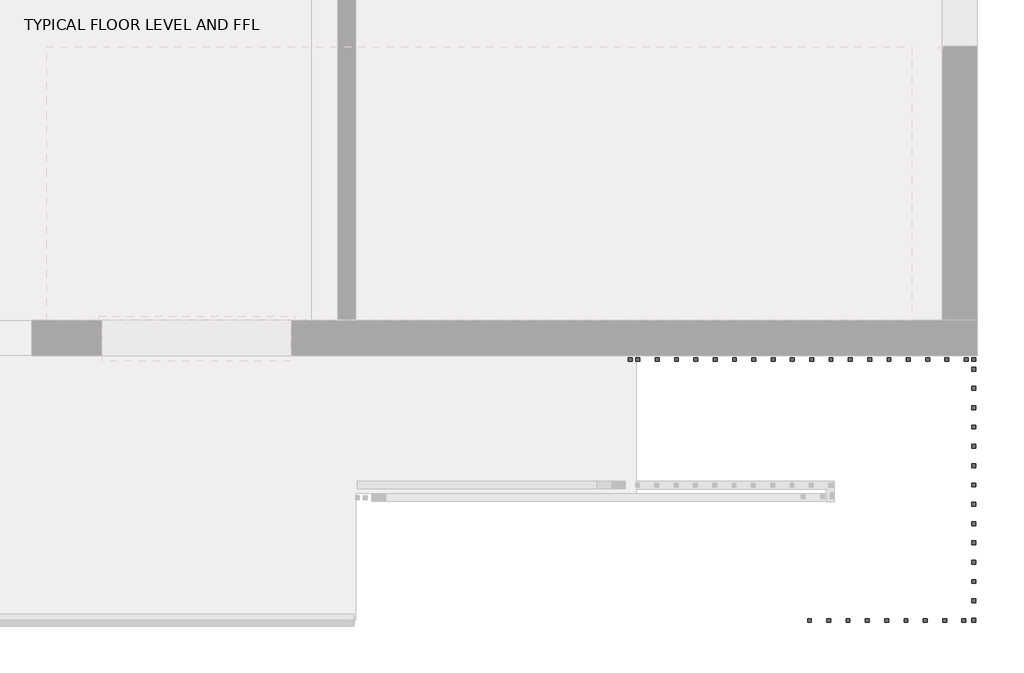
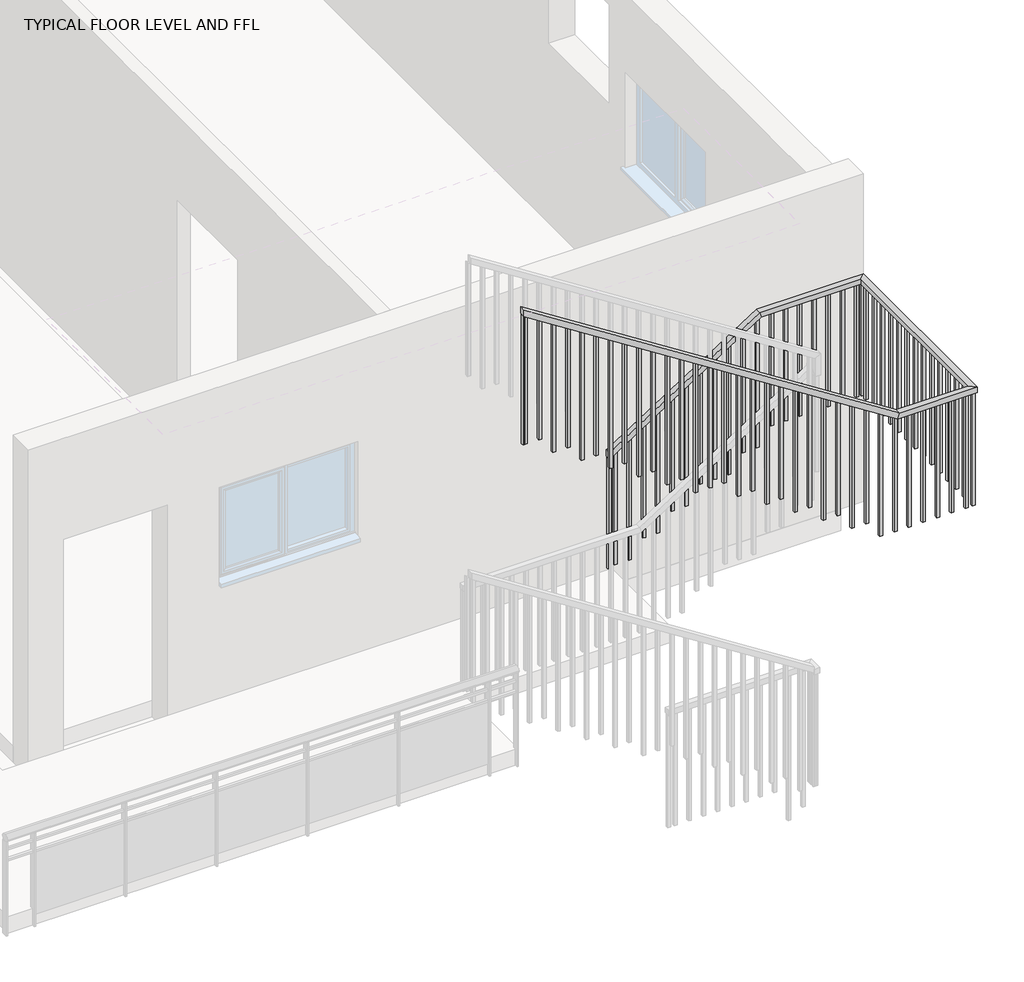
# One storey, part 2 of 3: 2 railings.
"""IFC4 building model written with IfcOpenShell, lengths in millimetres."""

from ifc_helpers import new_model, si_unit, frame, origin, place, context, project, spatial, polyline, outline, extrude, faceted_brep, element, save

model = new_model("IFC4")

# Units and contexts
model_context = context("Model", 3, world=origin())
ifc_project = project(units=[si_unit("LENGTHUNIT", "METRE", prefix="MILLI")], contexts=[model_context])

# Site, building, storey
site = spatial("IfcSite", under=ifc_project)
building = spatial("IfcBuilding", under=site)
storey = spatial("IfcBuildingStorey", under=building, Name="TYPICAL FLOOR LEVEL AND FFL", Elevation=3535.68)

# Railings
placement = place(None, origin())
element("IfcRailing", 1, ObjectType="1100mm", at=placement, inside=storey, context=model_context, shape_type="SolidModel", body=[
    faceted_brep([(-10457.8773536, -11114.0601959, 4838.88), (-10457.8773536, -11114.0601959, 4779.5164137), (-10457.8773536, -11164.0601959, 4779.5164137), (-10457.8773536, -11164.0601959, 4838.88), (-7447.5340108, -11114.0601959, 2912.2269781), (-7447.5340108, -11164.0601959, 2912.2269781), (-7447.5340108, -11164.0601959, 2852.8633918), (-7447.5340108, -11114.0601959, 2852.8633918)], [[[0, 1, 2, 3]], [[4, 5, 6, 7]], [[1, 0, 4, 7]], [[2, 1, 7, 6]], [[3, 2, 6, 5]], [[0, 3, 5, 4]]]),
    faceted_brep([(-7447.5340108, -11164.0601959, 2888.16), (-7447.5340108, -11164.0601959, 2838.16), (-7397.5340108, -11164.0601959, 2838.16), (-7397.5340108, -11164.0601959, 2888.16), (-7447.5340108, -11083.3255223, 2888.16), (-7447.5340108, -11083.3255223, 2838.16), (-7397.5340108, -11033.3255223, 2838.16), (-7397.5340108, -11033.3255223, 2888.16), (-8680.149573, -11083.3255223, 2888.16), (-8680.149573, -11033.3255223, 2888.16), (-8680.149573, -11033.3255223, 2838.16), (-8680.149573, -11083.3255223, 2838.16)], [[[0, 1, 2, 3]], [[1, 0, 4, 5]], [[2, 1, 5, 6]], [[3, 2, 6, 7]], [[0, 3, 7, 4]], [[8, 9, 10, 11]], [[5, 4, 8, 11]], [[6, 5, 11, 10]], [[7, 6, 10, 9]], [[4, 7, 9, 8]]]),
    extrude(outline(polyline([(-8597.5340108, -11045.8255223), (-8597.5340108, -11070.8255223), (-8622.5340108, -11070.8255223), (-8622.5340108, -11045.8255223), (-8597.5340108, -11045.8255223)])), frame((0.0, 0.0, 1788.16), z_axis=(0.0, 0.0, 1.0), x_axis=(1.0, 0.0, 0.0)), (0.0, 0.0, 1.0), 1050.0),
    extrude(outline(polyline([(-8472.5340108, -11045.8255223), (-8472.5340108, -11070.8255223), (-8497.5340108, -11070.8255223), (-8497.5340108, -11045.8255223), (-8472.5340108, -11045.8255223)])), frame((0.0, 0.0, 1788.16), z_axis=(0.0, 0.0, 1.0), x_axis=(1.0, 0.0, 0.0)), (0.0, 0.0, 1.0), 1050.0),
    extrude(outline(polyline([(-8347.5340108, -11045.8255223), (-8347.5340108, -11070.8255223), (-8372.5340108, -11070.8255223), (-8372.5340108, -11045.8255223), (-8347.5340108, -11045.8255223)])), frame((0.0, 0.0, 1788.16), z_axis=(0.0, 0.0, 1.0), x_axis=(1.0, 0.0, 0.0)), (0.0, 0.0, 1.0), 1050.0),
    extrude(outline(polyline([(-8222.5340108, -11045.8255223), (-8222.5340108, -11070.8255223), (-8247.5340108, -11070.8255223), (-8247.5340108, -11045.8255223), (-8222.5340108, -11045.8255223)])), frame((0.0, 0.0, 1788.16), z_axis=(0.0, 0.0, 1.0), x_axis=(1.0, 0.0, 0.0)), (0.0, 0.0, 1.0), 1050.0),
    extrude(outline(polyline([(-8097.5340108, -11045.8255223), (-8097.5340108, -11070.8255223), (-8122.5340108, -11070.8255223), (-8122.5340108, -11045.8255223), (-8097.5340108, -11045.8255223)])), frame((0.0, 0.0, 1788.16), z_axis=(0.0, 0.0, 1.0), x_axis=(1.0, 0.0, 0.0)), (0.0, 0.0, 1.0), 1050.0),
    extrude(outline(polyline([(-7972.5340108, -11045.8255223), (-7972.5340108, -11070.8255223), (-7997.5340108, -11070.8255223), (-7997.5340108, -11045.8255223), (-7972.5340108, -11045.8255223)])), frame((0.0, 0.0, 1788.16), z_axis=(0.0, 0.0, 1.0), x_axis=(1.0, 0.0, 0.0)), (0.0, 0.0, 1.0), 1050.0),
    extrude(outline(polyline([(-7847.5340108, -11045.8255223), (-7847.5340108, -11070.8255223), (-7872.5340108, -11070.8255223), (-7872.5340108, -11045.8255223), (-7847.5340108, -11045.8255223)])), frame((0.0, 0.0, 1788.16), z_axis=(0.0, 0.0, 1.0), x_axis=(1.0, 0.0, 0.0)), (0.0, 0.0, 1.0), 1050.0),
    extrude(outline(polyline([(-7722.5340108, -11045.8255223), (-7722.5340108, -11070.8255223), (-7747.5340108, -11070.8255223), (-7747.5340108, -11045.8255223), (-7722.5340108, -11045.8255223)])), frame((0.0, 0.0, 1788.16), z_axis=(0.0, 0.0, 1.0), x_axis=(1.0, 0.0, 0.0)), (0.0, 0.0, 1.0), 1050.0),
    extrude(outline(polyline([(-7597.5340108, -11045.8255223), (-7597.5340108, -11070.8255223), (-7622.5340108, -11070.8255223), (-7622.5340108, -11045.8255223), (-7597.5340108, -11045.8255223)])), frame((0.0, 0.0, 1484.4784954), z_axis=(0.0, 0.0, 1.0), x_axis=(1.0, 0.0, 0.0)), (0.0, 0.0, 1.0), 1353.6815046),
    extrude(outline(polyline([(-7472.5340108, -11045.8255223), (-7472.5340108, -11070.8255223), (-7497.5340108, -11070.8255223), (-7497.5340108, -11045.8255223), (-7472.5340108, -11045.8255223)])), frame((0.0, 0.0, 1564.4608651), z_axis=(0.0, 0.0, 1.0), x_axis=(1.0, 0.0, 0.0)), (0.0, 0.0, 1.0), 1273.6991349),
    extrude(outline(polyline([(-7410.0340108, -11089.0601959), (-7435.0340108, -11089.0601959), (-7435.0340108, -11064.0601959), (-7410.0340108, -11064.0601959), (-7410.0340108, -11089.0601959)])), frame((0.0, 0.0, 1770.6), z_axis=(0.0, 0.0, 1.0), x_axis=(1.0, 0.0, 0.0)), (0.0, 0.0, 1.0), 1067.56),
    extrude(outline(polyline([(2851.8393741, -7445.9340108), (1788.16, -7445.9340108), (1788.16, -7420.9340108), (2835.8390977, -7420.9340108), (2851.8393741, -7445.9340108)])), frame((0.0, -11151.5601959, 0.0), z_axis=(0.0, 1.0, 0.0), x_axis=(0.0, 0.0, 1.0)), (0.0, 0.0, 1.0), 25.0),
    extrude(outline(polyline([(2931.8407561, -7570.9340108), (1788.16, -7570.9340108), (1788.16, -7545.9340108), (2915.8404797, -7545.9340108), (2931.8407561, -7570.9340108)])), frame((0.0, -11151.5601959, 0.0), z_axis=(0.0, 1.0, 0.0), x_axis=(0.0, 0.0, 1.0)), (0.0, 0.0, 1.0), 25.0),
    extrude(outline(polyline([(3011.8421381, -7695.9340108), (1950.72, -7695.9340108), (1950.72, -7670.9340108), (2995.8418617, -7670.9340108), (3011.8421381, -7695.9340108)])), frame((0.0, -11151.5601959, 0.0), z_axis=(0.0, 1.0, 0.0), x_axis=(0.0, 0.0, 1.0)), (0.0, 0.0, 1.0), 25.0),
    extrude(outline(polyline([(3091.8435201, -7820.9340108), (1950.72, -7820.9340108), (1950.72, -7795.9340108), (3075.8432437, -7795.9340108), (3091.8435201, -7820.9340108)])), frame((0.0, -11151.5601959, 0.0), z_axis=(0.0, 1.0, 0.0), x_axis=(0.0, 0.0, 1.0)), (0.0, 0.0, 1.0), 25.0),
    extrude(outline(polyline([(3171.8449021, -7945.9340108), (2113.28, -7945.9340108), (2113.28, -7920.9340108), (3155.8446257, -7920.9340108), (3171.8449021, -7945.9340108)])), frame((0.0, -11151.5601959, 0.0), z_axis=(0.0, 1.0, 0.0), x_axis=(0.0, 0.0, 1.0)), (0.0, 0.0, 1.0), 25.0),
    extrude(outline(polyline([(3251.8462841, -8070.9340108), (2113.28, -8070.9340108), (2113.28, -8045.9340108), (3235.8460077, -8045.9340108), (3251.8462841, -8070.9340108)])), frame((0.0, -11151.5601959, 0.0), z_axis=(0.0, 1.0, 0.0), x_axis=(0.0, 0.0, 1.0)), (0.0, 0.0, 1.0), 25.0),
    extrude(outline(polyline([(3331.8476661, -8195.9340108), (2275.84, -8195.9340108), (2275.84, -8170.9340108), (3315.8473897, -8170.9340108), (3331.8476661, -8195.9340108)])), frame((0.0, -11151.5601959, 0.0), z_axis=(0.0, 1.0, 0.0), x_axis=(0.0, 0.0, 1.0)), (0.0, 0.0, 1.0), 25.0),
    extrude(outline(polyline([(3411.8490481, -8320.9340108), (2275.84, -8320.9340108), (2275.84, -8295.9340108), (3395.8487717, -8295.9340108), (3411.8490481, -8320.9340108)])), frame((0.0, -11151.5601959, 0.0), z_axis=(0.0, 1.0, 0.0), x_axis=(0.0, 0.0, 1.0)), (0.0, 0.0, 1.0), 25.0),
    extrude(outline(polyline([(3491.8504301, -8445.9340108), (2438.4, -8445.9340108), (2438.4, -8420.9340108), (3475.8501537, -8420.9340108), (3491.8504301, -8445.9340108)])), frame((0.0, -11151.5601959, 0.0), z_axis=(0.0, 1.0, 0.0), x_axis=(0.0, 0.0, 1.0)), (0.0, 0.0, 1.0), 25.0),
    extrude(outline(polyline([(3571.8518121, -8570.9340108), (2438.4, -8570.9340108), (2438.4, -8545.9340108), (3555.8515357, -8545.9340108), (3571.8518121, -8570.9340108)])), frame((0.0, -11151.5601959, 0.0), z_axis=(0.0, 1.0, 0.0), x_axis=(0.0, 0.0, 1.0)), (0.0, 0.0, 1.0), 25.0),
    extrude(outline(polyline([(3651.8531942, -8695.9340108), (2600.96, -8695.9340108), (2600.96, -8670.9340108), (3635.8529178, -8670.9340108), (3651.8531942, -8695.9340108)])), frame((0.0, -11151.5601959, 0.0), z_axis=(0.0, 1.0, 0.0), x_axis=(0.0, 0.0, 1.0)), (0.0, 0.0, 1.0), 25.0),
    extrude(outline(polyline([(3731.8545762, -8820.9340108), (2600.96, -8820.9340108), (2600.96, -8795.9340108), (3715.8542998, -8795.9340108), (3731.8545762, -8820.9340108)])), frame((0.0, -11151.5601959, 0.0), z_axis=(0.0, 1.0, 0.0), x_axis=(0.0, 0.0, 1.0)), (0.0, 0.0, 1.0), 25.0),
    extrude(outline(polyline([(3811.8559582, -8945.9340108), (2600.96, -8945.9340108), (2600.96, -8920.9340108), (3795.8556818, -8920.9340108), (3811.8559582, -8945.9340108)])), frame((0.0, -11151.5601959, 0.0), z_axis=(0.0, 1.0, 0.0), x_axis=(0.0, 0.0, 1.0)), (0.0, 0.0, 1.0), 25.0),
    extrude(outline(polyline([(3891.8573402, -9070.9340108), (2763.52, -9070.9340108), (2763.52, -9045.9340108), (3875.8570638, -9045.9340108), (3891.8573402, -9070.9340108)])), frame((0.0, -11151.5601959, 0.0), z_axis=(0.0, 1.0, 0.0), x_axis=(0.0, 0.0, 1.0)), (0.0, 0.0, 1.0), 25.0),
    extrude(outline(polyline([(3971.8587222, -9195.9340108), (2763.52, -9195.9340108), (2763.52, -9170.9340108), (3955.8584458, -9170.9340108), (3971.8587222, -9195.9340108)])), frame((0.0, -11151.5601959, 0.0), z_axis=(0.0, 1.0, 0.0), x_axis=(0.0, 0.0, 1.0)), (0.0, 0.0, 1.0), 25.0),
    extrude(outline(polyline([(4051.8601042, -9320.9340108), (2926.08, -9320.9340108), (2926.08, -9295.9340108), (4035.8598278, -9295.9340108), (4051.8601042, -9320.9340108)])), frame((0.0, -11151.5601959, 0.0), z_axis=(0.0, 1.0, 0.0), x_axis=(0.0, 0.0, 1.0)), (0.0, 0.0, 1.0), 25.0),
    extrude(outline(polyline([(4131.8614862, -9445.9340108), (2926.08, -9445.9340108), (2926.08, -9420.9340108), (4115.8612098, -9420.9340108), (4131.8614862, -9445.9340108)])), frame((0.0, -11151.5601959, 0.0), z_axis=(0.0, 1.0, 0.0), x_axis=(0.0, 0.0, 1.0)), (0.0, 0.0, 1.0), 25.0),
    extrude(outline(polyline([(4211.8628682, -9570.9340108), (3088.64, -9570.9340108), (3088.64, -9545.9340108), (4195.8625918, -9545.9340108), (4211.8628682, -9570.9340108)])), frame((0.0, -11151.5601959, 0.0), z_axis=(0.0, 1.0, 0.0), x_axis=(0.0, 0.0, 1.0)), (0.0, 0.0, 1.0), 25.0),
    extrude(outline(polyline([(4291.8642502, -9695.9340108), (3088.64, -9695.9340108), (3088.64, -9670.9340108), (4275.8639738, -9670.9340108), (4291.8642502, -9695.9340108)])), frame((0.0, -11151.5601959, 0.0), z_axis=(0.0, 1.0, 0.0), x_axis=(0.0, 0.0, 1.0)), (0.0, 0.0, 1.0), 25.0),
    extrude(outline(polyline([(4371.8656322, -9820.9340108), (3251.2, -9820.9340108), (3251.2, -9795.9340108), (4355.8653558, -9795.9340108), (4371.8656322, -9820.9340108)])), frame((0.0, -11151.5601959, 0.0), z_axis=(0.0, 1.0, 0.0), x_axis=(0.0, 0.0, 1.0)), (0.0, 0.0, 1.0), 25.0),
    extrude(outline(polyline([(4451.8670143, -9945.9340108), (3251.2, -9945.9340108), (3251.2, -9920.9340108), (4435.8667379, -9920.9340108), (4451.8670143, -9945.9340108)])), frame((0.0, -11151.5601959, 0.0), z_axis=(0.0, 1.0, 0.0), x_axis=(0.0, 0.0, 1.0)), (0.0, 0.0, 1.0), 25.0),
    extrude(outline(polyline([(4531.8683963, -10070.9340108), (3413.76, -10070.9340108), (3413.76, -10045.9340108), (4515.8681199, -10045.9340108), (4531.8683963, -10070.9340108)])), frame((0.0, -11151.5601959, 0.0), z_axis=(0.0, 1.0, 0.0), x_axis=(0.0, 0.0, 1.0)), (0.0, 0.0, 1.0), 25.0),
    extrude(outline(polyline([(4611.8697783, -10195.9340108), (3413.76, -10195.9340108), (3413.76, -10170.9340108), (4595.8695019, -10170.9340108), (4611.8697783, -10195.9340108)])), frame((0.0, -11151.5601959, 0.0), z_axis=(0.0, 1.0, 0.0), x_axis=(0.0, 0.0, 1.0)), (0.0, 0.0, 1.0), 25.0),
    extrude(outline(polyline([(4691.8711603, -10320.9340108), (3576.32, -10320.9340108), (3576.32, -10295.9340108), (4675.8708839, -10295.9340108), (4691.8711603, -10320.9340108)])), frame((0.0, -11151.5601959, 0.0), z_axis=(0.0, 1.0, 0.0), x_axis=(0.0, 0.0, 1.0)), (0.0, 0.0, 1.0), 25.0),
    extrude(outline(polyline([(4771.8725423, -10445.9340108), (3576.32, -10445.9340108), (3576.32, -10420.9340108), (4755.8722659, -10420.9340108), (4771.8725423, -10445.9340108)])), frame((0.0, -11151.5601959, 0.0), z_axis=(0.0, 1.0, 0.0), x_axis=(0.0, 0.0, 1.0)), (0.0, 0.0, 1.0), 25.0),
    extrude(outline(polyline([(-7410.0340108, -11070.8255223), (-7435.0340108, -11070.8255223), (-7435.0340108, -11045.8255223), (-7410.0340108, -11045.8255223), (-7410.0340108, -11070.8255223)])), frame((0.0, 0.0, 1770.6), z_axis=(0.0, 0.0, 1.0), x_axis=(1.0, 0.0, 0.0)), (0.0, 0.0, 1.0), 1067.56),
    extrude(outline(polyline([(2844.8632536, -7435.0340108), (1788.16, -7435.0340108), (1788.16, -7410.0340108), (2828.8629772, -7410.0340108), (2844.8632536, -7435.0340108)])), frame((0.0, -11151.5601959, 0.0), z_axis=(0.0, 1.0, 0.0), x_axis=(0.0, 0.0, 1.0)), (0.0, 0.0, 1.0), 25.0),
    extrude(outline(polyline([(-8655.149573, -11045.8255223), (-8655.149573, -11070.8255223), (-8680.149573, -11070.8255223), (-8680.149573, -11045.8255223), (-8655.149573, -11045.8255223)])), frame((0.0, 0.0, 1788.16), z_axis=(0.0, 0.0, 1.0), x_axis=(1.0, 0.0, 0.0)), (0.0, 0.0, 1.0), 1050.0),
    extrude(outline(polyline([(4803.8730951, -10495.9340108), (3738.88, -10495.9340108), (3738.88, -10470.9340108), (4787.8728187, -10470.9340108), (4803.8730951, -10495.9340108)])), frame((0.0, -11151.5601959, 0.0), z_axis=(0.0, 1.0, 0.0), x_axis=(0.0, 0.0, 1.0)), (0.0, 0.0, 1.0), 25.0),
])
element("IfcRailing", 2, ObjectType="1100mm", at=placement, inside=storey, context=model_context, shape_type="SolidModel", body=[
    faceted_brep([(-8730.6132565, -10219.6521308, 4806.5938931), (-8730.6132565, -10219.6521308, 4747.2362925), (-8730.6132565, -10269.6521308, 4747.2362925), (-8730.6132565, -10269.6521308, 4806.5938931), (-7409.7306254, -10219.6521308, 5651.68), (-7395.1045513, -10219.6521308, 5601.68), (-7395.1045513, -10269.6521308, 5601.68), (-7409.7306254, -10269.6521308, 5651.68), (-6470.4132565, -10219.6521308, 5601.68), (-6470.4132565, -10219.6521308, 5651.68), (-6470.4132565, -11959.0860066, 5651.68), (-6470.4132565, -11959.0860066, 5601.68), (-6520.4132565, -10269.6521308, 5601.68), (-6520.4132565, -11909.0860066, 5601.68), (-6520.4132565, -10269.6521308, 5651.68), (-6520.4132565, -11909.0860066, 5651.68), (-7155.7350132, -11959.0860066, 5651.68), (-7170.3653641, -11959.0860066, 5601.68), (-7170.3653641, -11909.0860066, 5601.68), (-7155.7350132, -11909.0860066, 5651.68), (-10457.8132565, -11959.0860066, 7765.0465838), (-10457.8132565, -11909.0860066, 7765.0465838), (-10457.8132565, -11909.0860066, 7705.6829974), (-10457.8132565, -11959.0860066, 7705.6829974)], [[[0, 1, 2, 3]], [[1, 0, 4, 5]], [[2, 1, 5, 6]], [[3, 2, 6, 7]], [[0, 3, 7, 4]], [[8, 9, 10, 11]], [[12, 8, 11, 13]], [[14, 12, 13, 15]], [[9, 14, 15, 10]], [[5, 4, 9, 8]], [[6, 5, 8, 12]], [[7, 6, 12, 14]], [[4, 7, 14, 9]], [[11, 10, 16, 17]], [[13, 11, 17, 18]], [[15, 13, 18, 19]], [[10, 15, 19, 16]], [[20, 21, 22, 23]], [[17, 16, 20, 23]], [[18, 17, 23, 22]], [[19, 18, 22, 21]], [[16, 19, 21, 20]]]),
    extrude(outline(polyline([(6502.4, -10420.4132565), (7681.746584, -10420.4132565), (7697.7468604, -10445.4132565), (6502.4, -10445.4132565), (6502.4, -10420.4132565)])), frame((0.0, -11946.5860066, 0.0), z_axis=(0.0, 1.0, 0.0), x_axis=(0.0, 0.0, 1.0)), (0.0, 0.0, 1.0), 25.0),
    extrude(outline(polyline([(6502.4, -10295.4132565), (7601.7452019, -10295.4132565), (7617.7454783, -10320.4132565), (6502.4, -10320.4132565), (6502.4, -10295.4132565)])), frame((0.0, -11946.5860066, 0.0), z_axis=(0.0, 1.0, 0.0), x_axis=(0.0, 0.0, 1.0)), (0.0, 0.0, 1.0), 25.0),
    extrude(outline(polyline([(6339.84, -10170.4132565), (7521.7438199, -10170.4132565), (7537.7440963, -10195.4132565), (6339.84, -10195.4132565), (6339.84, -10170.4132565)])), frame((0.0, -11946.5860066, 0.0), z_axis=(0.0, 1.0, 0.0), x_axis=(0.0, 0.0, 1.0)), (0.0, 0.0, 1.0), 25.0),
    extrude(outline(polyline([(6339.84, -10045.4132565), (7441.7424379, -10045.4132565), (7457.7427143, -10070.4132565), (6339.84, -10070.4132565), (6339.84, -10045.4132565)])), frame((0.0, -11946.5860066, 0.0), z_axis=(0.0, 1.0, 0.0), x_axis=(0.0, 0.0, 1.0)), (0.0, 0.0, 1.0), 25.0),
    extrude(outline(polyline([(6177.28, -9920.4132565), (7361.7410559, -9920.4132565), (7377.7413323, -9945.4132565), (6177.28, -9945.4132565), (6177.28, -9920.4132565)])), frame((0.0, -11946.5860066, 0.0), z_axis=(0.0, 1.0, 0.0), x_axis=(0.0, 0.0, 1.0)), (0.0, 0.0, 1.0), 25.0),
    extrude(outline(polyline([(6177.28, -9795.4132565), (7281.7396739, -9795.4132565), (7297.7399503, -9820.4132565), (6177.28, -9820.4132565), (6177.28, -9795.4132565)])), frame((0.0, -11946.5860066, 0.0), z_axis=(0.0, 1.0, 0.0), x_axis=(0.0, 0.0, 1.0)), (0.0, 0.0, 1.0), 25.0),
    extrude(outline(polyline([(6014.72, -9670.4132565), (7201.7382919, -9670.4132565), (7217.7385683, -9695.4132565), (6014.72, -9695.4132565), (6014.72, -9670.4132565)])), frame((0.0, -11946.5860066, 0.0), z_axis=(0.0, 1.0, 0.0), x_axis=(0.0, 0.0, 1.0)), (0.0, 0.0, 1.0), 25.0),
    extrude(outline(polyline([(6014.72, -9545.4132565), (7121.7369099, -9545.4132565), (7137.7371863, -9570.4132565), (6014.72, -9570.4132565), (6014.72, -9545.4132565)])), frame((0.0, -11946.5860066, 0.0), z_axis=(0.0, 1.0, 0.0), x_axis=(0.0, 0.0, 1.0)), (0.0, 0.0, 1.0), 25.0),
    extrude(outline(polyline([(5852.16, -9420.4132565), (7041.7355279, -9420.4132565), (7057.7358043, -9445.4132565), (5852.16, -9445.4132565), (5852.16, -9420.4132565)])), frame((0.0, -11946.5860066, 0.0), z_axis=(0.0, 1.0, 0.0), x_axis=(0.0, 0.0, 1.0)), (0.0, 0.0, 1.0), 25.0),
    extrude(outline(polyline([(5852.16, -9295.4132565), (6961.7341459, -9295.4132565), (6977.7344223, -9320.4132565), (5852.16, -9320.4132565), (5852.16, -9295.4132565)])), frame((0.0, -11946.5860066, 0.0), z_axis=(0.0, 1.0, 0.0), x_axis=(0.0, 0.0, 1.0)), (0.0, 0.0, 1.0), 25.0),
    extrude(outline(polyline([(5689.6, -9170.4132565), (6881.7327639, -9170.4132565), (6897.7330403, -9195.4132565), (5689.6, -9195.4132565), (5689.6, -9170.4132565)])), frame((0.0, -11946.5860066, 0.0), z_axis=(0.0, 1.0, 0.0), x_axis=(0.0, 0.0, 1.0)), (0.0, 0.0, 1.0), 25.0),
    extrude(outline(polyline([(5689.6, -9045.4132565), (6801.7313818, -9045.4132565), (6817.7316582, -9070.4132565), (5689.6, -9070.4132565), (5689.6, -9045.4132565)])), frame((0.0, -11946.5860066, 0.0), z_axis=(0.0, 1.0, 0.0), x_axis=(0.0, 0.0, 1.0)), (0.0, 0.0, 1.0), 25.0),
    extrude(outline(polyline([(5527.04, -8920.4132565), (6721.7299998, -8920.4132565), (6737.7302762, -8945.4132565), (5527.04, -8945.4132565), (5527.04, -8920.4132565)])), frame((0.0, -11946.5860066, 0.0), z_axis=(0.0, 1.0, 0.0), x_axis=(0.0, 0.0, 1.0)), (0.0, 0.0, 1.0), 25.0),
    extrude(outline(polyline([(5527.04, -8795.4132565), (6641.7286178, -8795.4132565), (6657.7288942, -8820.4132565), (5527.04, -8820.4132565), (5527.04, -8795.4132565)])), frame((0.0, -11946.5860066, 0.0), z_axis=(0.0, 1.0, 0.0), x_axis=(0.0, 0.0, 1.0)), (0.0, 0.0, 1.0), 25.0),
    extrude(outline(polyline([(5527.04, -8670.4132565), (6561.7272358, -8670.4132565), (6577.7275122, -8695.4132565), (5527.04, -8695.4132565), (5527.04, -8670.4132565)])), frame((0.0, -11946.5860066, 0.0), z_axis=(0.0, 1.0, 0.0), x_axis=(0.0, 0.0, 1.0)), (0.0, 0.0, 1.0), 25.0),
    extrude(outline(polyline([(5364.48, -8545.4132565), (6481.7258538, -8545.4132565), (6497.7261302, -8570.4132565), (5364.48, -8570.4132565), (5364.48, -8545.4132565)])), frame((0.0, -11946.5860066, 0.0), z_axis=(0.0, 1.0, 0.0), x_axis=(0.0, 0.0, 1.0)), (0.0, 0.0, 1.0), 25.0),
    extrude(outline(polyline([(5364.48, -8420.4132565), (6401.7244718, -8420.4132565), (6417.7247482, -8445.4132565), (5364.48, -8445.4132565), (5364.48, -8420.4132565)])), frame((0.0, -11946.5860066, 0.0), z_axis=(0.0, 1.0, 0.0), x_axis=(0.0, 0.0, 1.0)), (0.0, 0.0, 1.0), 25.0),
    extrude(outline(polyline([(5201.92, -8295.4132565), (6321.7230898, -8295.4132565), (6337.7233662, -8320.4132565), (5201.92, -8320.4132565), (5201.92, -8295.4132565)])), frame((0.0, -11946.5860066, 0.0), z_axis=(0.0, 1.0, 0.0), x_axis=(0.0, 0.0, 1.0)), (0.0, 0.0, 1.0), 25.0),
    extrude(outline(polyline([(5201.92, -8170.4132565), (6241.7217078, -8170.4132565), (6257.7219842, -8195.4132565), (5201.92, -8195.4132565), (5201.92, -8170.4132565)])), frame((0.0, -11946.5860066, 0.0), z_axis=(0.0, 1.0, 0.0), x_axis=(0.0, 0.0, 1.0)), (0.0, 0.0, 1.0), 25.0),
    extrude(outline(polyline([(5039.36, -8045.4132565), (6161.7203258, -8045.4132565), (6177.7206022, -8070.4132565), (5039.36, -8070.4132565), (5039.36, -8045.4132565)])), frame((0.0, -11946.5860066, 0.0), z_axis=(0.0, 1.0, 0.0), x_axis=(0.0, 0.0, 1.0)), (0.0, 0.0, 1.0), 25.0),
    extrude(outline(polyline([(5039.36, -7920.4132565), (6081.7189438, -7920.4132565), (6097.7192202, -7945.4132565), (5039.36, -7945.4132565), (5039.36, -7920.4132565)])), frame((0.0, -11946.5860066, 0.0), z_axis=(0.0, 1.0, 0.0), x_axis=(0.0, 0.0, 1.0)), (0.0, 0.0, 1.0), 25.0),
    extrude(outline(polyline([(4876.8, -7795.4132565), (6001.7175618, -7795.4132565), (6017.7178382, -7820.4132565), (4876.8, -7820.4132565), (4876.8, -7795.4132565)])), frame((0.0, -11946.5860066, 0.0), z_axis=(0.0, 1.0, 0.0), x_axis=(0.0, 0.0, 1.0)), (0.0, 0.0, 1.0), 25.0),
    extrude(outline(polyline([(4876.8, -7670.4132565), (5921.7161797, -7670.4132565), (5937.7164561, -7695.4132565), (4876.8, -7695.4132565), (4876.8, -7670.4132565)])), frame((0.0, -11946.5860066, 0.0), z_axis=(0.0, 1.0, 0.0), x_axis=(0.0, 0.0, 1.0)), (0.0, 0.0, 1.0), 25.0),
    extrude(outline(polyline([(4714.24, -7545.4132565), (5841.7147977, -7545.4132565), (5857.7150741, -7570.4132565), (4714.24, -7570.4132565), (4714.24, -7545.4132565)])), frame((0.0, -11946.5860066, 0.0), z_axis=(0.0, 1.0, 0.0), x_axis=(0.0, 0.0, 1.0)), (0.0, 0.0, 1.0), 25.0),
    extrude(outline(polyline([(4714.24, -7420.4132565), (5761.7134157, -7420.4132565), (5777.7136921, -7445.4132565), (4714.24, -7445.4132565), (4714.24, -7420.4132565)])), frame((0.0, -11946.5860066, 0.0), z_axis=(0.0, 1.0, 0.0), x_axis=(0.0, 0.0, 1.0)), (0.0, 0.0, 1.0), 25.0),
    extrude(outline(polyline([(4551.68, -7295.4132565), (5681.7120337, -7295.4132565), (5697.7123101, -7320.4132565), (4551.68, -7320.4132565), (4551.68, -7295.4132565)])), frame((0.0, -11946.5860066, 0.0), z_axis=(0.0, 1.0, 0.0), x_axis=(0.0, 0.0, 1.0)), (0.0, 0.0, 1.0), 25.0),
    extrude(outline(polyline([(4551.68, -7170.4132565), (5601.7106517, -7170.4132565), (5617.7109281, -7195.4132565), (4551.68, -7195.4132565), (4551.68, -7170.4132565)])), frame((0.0, -11946.5860066, 0.0), z_axis=(0.0, 1.0, 0.0), x_axis=(0.0, 0.0, 1.0)), (0.0, 0.0, 1.0), 25.0),
    extrude(outline(polyline([(-7045.4132565, -11921.5860066), (-7045.4132565, -11946.5860066), (-7070.4132565, -11946.5860066), (-7070.4132565, -11921.5860066), (-7045.4132565, -11921.5860066)])), frame((0.0, 0.0, 4551.68), z_axis=(0.0, 0.0, 1.0), x_axis=(1.0, 0.0, 0.0)), (0.0, 0.0, 1.0), 1050.0),
    extrude(outline(polyline([(-6920.4132565, -11921.5860066), (-6920.4132565, -11946.5860066), (-6945.4132565, -11946.5860066), (-6945.4132565, -11921.5860066), (-6920.4132565, -11921.5860066)])), frame((0.0, 0.0, 4551.68), z_axis=(0.0, 0.0, 1.0), x_axis=(1.0, 0.0, 0.0)), (0.0, 0.0, 1.0), 1050.0),
    extrude(outline(polyline([(-6795.4132565, -11921.5860066), (-6795.4132565, -11946.5860066), (-6820.4132565, -11946.5860066), (-6820.4132565, -11921.5860066), (-6795.4132565, -11921.5860066)])), frame((0.0, 0.0, 4551.68), z_axis=(0.0, 0.0, 1.0), x_axis=(1.0, 0.0, 0.0)), (0.0, 0.0, 1.0), 1050.0),
    extrude(outline(polyline([(-6670.4132565, -11921.5860066), (-6670.4132565, -11946.5860066), (-6695.4132565, -11946.5860066), (-6695.4132565, -11921.5860066), (-6670.4132565, -11921.5860066)])), frame((0.0, 0.0, 4551.68), z_axis=(0.0, 0.0, 1.0), x_axis=(1.0, 0.0, 0.0)), (0.0, 0.0, 1.0), 1050.0),
    extrude(outline(polyline([(-6545.4132565, -11921.5860066), (-6545.4132565, -11946.5860066), (-6570.4132565, -11946.5860066), (-6570.4132565, -11921.5860066), (-6545.4132565, -11921.5860066)])), frame((0.0, 0.0, 4551.68), z_axis=(0.0, 0.0, 1.0), x_axis=(1.0, 0.0, 0.0)), (0.0, 0.0, 1.0), 1050.0),
    extrude(outline(polyline([(-6507.9132565, -11919.6521308), (-6482.9132565, -11919.6521308), (-6482.9132565, -11944.6521308), (-6507.9132565, -11944.6521308), (-6507.9132565, -11919.6521308)])), frame((0.0, 0.0, 4551.68), z_axis=(0.0, 0.0, 1.0), x_axis=(1.0, 0.0, 0.0)), (0.0, 0.0, 1.0), 1050.0),
    extrude(outline(polyline([(-6507.9132565, -11794.6521308), (-6482.9132565, -11794.6521308), (-6482.9132565, -11819.6521308), (-6507.9132565, -11819.6521308), (-6507.9132565, -11794.6521308)])), frame((0.0, 0.0, 4551.68), z_axis=(0.0, 0.0, 1.0), x_axis=(1.0, 0.0, 0.0)), (0.0, 0.0, 1.0), 1050.0),
    extrude(outline(polyline([(-6507.9132565, -11669.6521308), (-6482.9132565, -11669.6521308), (-6482.9132565, -11694.6521308), (-6507.9132565, -11694.6521308), (-6507.9132565, -11669.6521308)])), frame((0.0, 0.0, 4551.68), z_axis=(0.0, 0.0, 1.0), x_axis=(1.0, 0.0, 0.0)), (0.0, 0.0, 1.0), 1050.0),
    extrude(outline(polyline([(-6507.9132565, -11544.6521308), (-6482.9132565, -11544.6521308), (-6482.9132565, -11569.6521308), (-6507.9132565, -11569.6521308), (-6507.9132565, -11544.6521308)])), frame((0.0, 0.0, 4551.68), z_axis=(0.0, 0.0, 1.0), x_axis=(1.0, 0.0, 0.0)), (0.0, 0.0, 1.0), 1050.0),
    extrude(outline(polyline([(-6507.9132565, -11419.6521308), (-6482.9132565, -11419.6521308), (-6482.9132565, -11444.6521308), (-6507.9132565, -11444.6521308), (-6507.9132565, -11419.6521308)])), frame((0.0, 0.0, 4551.68), z_axis=(0.0, 0.0, 1.0), x_axis=(1.0, 0.0, 0.0)), (0.0, 0.0, 1.0), 1050.0),
    extrude(outline(polyline([(-6507.9132565, -11294.6521308), (-6482.9132565, -11294.6521308), (-6482.9132565, -11319.6521308), (-6507.9132565, -11319.6521308), (-6507.9132565, -11294.6521308)])), frame((0.0, 0.0, 4551.68), z_axis=(0.0, 0.0, 1.0), x_axis=(1.0, 0.0, 0.0)), (0.0, 0.0, 1.0), 1050.0),
    extrude(outline(polyline([(-6507.9132565, -11169.6521308), (-6482.9132565, -11169.6521308), (-6482.9132565, -11194.6521308), (-6507.9132565, -11194.6521308), (-6507.9132565, -11169.6521308)])), frame((0.0, 0.0, 4551.68), z_axis=(0.0, 0.0, 1.0), x_axis=(1.0, 0.0, 0.0)), (0.0, 0.0, 1.0), 1050.0),
    extrude(outline(polyline([(-6507.9132565, -11044.6521308), (-6482.9132565, -11044.6521308), (-6482.9132565, -11069.6521308), (-6507.9132565, -11069.6521308), (-6507.9132565, -11044.6521308)])), frame((0.0, 0.0, 4551.68), z_axis=(0.0, 0.0, 1.0), x_axis=(1.0, 0.0, 0.0)), (0.0, 0.0, 1.0), 1050.0),
    extrude(outline(polyline([(-6507.9132565, -10919.6521308), (-6482.9132565, -10919.6521308), (-6482.9132565, -10944.6521308), (-6507.9132565, -10944.6521308), (-6507.9132565, -10919.6521308)])), frame((0.0, 0.0, 4551.68), z_axis=(0.0, 0.0, 1.0), x_axis=(1.0, 0.0, 0.0)), (0.0, 0.0, 1.0), 1050.0),
    extrude(outline(polyline([(-6507.9132565, -10794.6521308), (-6482.9132565, -10794.6521308), (-6482.9132565, -10819.6521308), (-6507.9132565, -10819.6521308), (-6507.9132565, -10794.6521308)])), frame((0.0, 0.0, 4551.68), z_axis=(0.0, 0.0, 1.0), x_axis=(1.0, 0.0, 0.0)), (0.0, 0.0, 1.0), 1050.0),
    extrude(outline(polyline([(-6507.9132565, -10669.6521308), (-6482.9132565, -10669.6521308), (-6482.9132565, -10694.6521308), (-6507.9132565, -10694.6521308), (-6507.9132565, -10669.6521308)])), frame((0.0, 0.0, 4551.68), z_axis=(0.0, 0.0, 1.0), x_axis=(1.0, 0.0, 0.0)), (0.0, 0.0, 1.0), 1050.0),
    extrude(outline(polyline([(-6507.9132565, -10544.6521308), (-6482.9132565, -10544.6521308), (-6482.9132565, -10569.6521308), (-6507.9132565, -10569.6521308), (-6507.9132565, -10544.6521308)])), frame((0.0, 0.0, 4551.68), z_axis=(0.0, 0.0, 1.0), x_axis=(1.0, 0.0, 0.0)), (0.0, 0.0, 1.0), 1050.0),
    extrude(outline(polyline([(-6507.9132565, -10419.6521308), (-6482.9132565, -10419.6521308), (-6482.9132565, -10444.6521308), (-6507.9132565, -10444.6521308), (-6507.9132565, -10419.6521308)])), frame((0.0, 0.0, 4551.68), z_axis=(0.0, 0.0, 1.0), x_axis=(1.0, 0.0, 0.0)), (0.0, 0.0, 1.0), 1050.0),
    extrude(outline(polyline([(-6507.9132565, -10294.6521308), (-6482.9132565, -10294.6521308), (-6482.9132565, -10319.6521308), (-6507.9132565, -10319.6521308), (-6507.9132565, -10294.6521308)])), frame((0.0, 0.0, 4551.68), z_axis=(0.0, 0.0, 1.0), x_axis=(1.0, 0.0, 0.0)), (0.0, 0.0, 1.0), 1050.0),
    extrude(outline(polyline([(-6555.6132565, -10257.1521308), (-6555.6132565, -10232.1521308), (-6530.6132565, -10232.1521308), (-6530.6132565, -10257.1521308), (-6555.6132565, -10257.1521308)])), frame((0.0, 0.0, 4551.68), z_axis=(0.0, 0.0, 1.0), x_axis=(1.0, 0.0, 0.0)), (0.0, 0.0, 1.0), 1050.0),
    extrude(outline(polyline([(-6680.6132565, -10257.1521308), (-6680.6132565, -10232.1521308), (-6655.6132565, -10232.1521308), (-6655.6132565, -10257.1521308), (-6680.6132565, -10257.1521308)])), frame((0.0, 0.0, 4551.68), z_axis=(0.0, 0.0, 1.0), x_axis=(1.0, 0.0, 0.0)), (0.0, 0.0, 1.0), 1050.0),
    extrude(outline(polyline([(-6805.6132565, -10257.1521308), (-6805.6132565, -10232.1521308), (-6780.6132565, -10232.1521308), (-6780.6132565, -10257.1521308), (-6805.6132565, -10257.1521308)])), frame((0.0, 0.0, 4551.68), z_axis=(0.0, 0.0, 1.0), x_axis=(1.0, 0.0, 0.0)), (0.0, 0.0, 1.0), 1050.0),
    extrude(outline(polyline([(-6930.6132565, -10257.1521308), (-6930.6132565, -10232.1521308), (-6905.6132565, -10232.1521308), (-6905.6132565, -10257.1521308), (-6930.6132565, -10257.1521308)])), frame((0.0, 0.0, 4551.68), z_axis=(0.0, 0.0, 1.0), x_axis=(1.0, 0.0, 0.0)), (0.0, 0.0, 1.0), 1050.0),
    extrude(outline(polyline([(-7055.6132565, -10257.1521308), (-7055.6132565, -10232.1521308), (-7030.6132565, -10232.1521308), (-7030.6132565, -10257.1521308), (-7055.6132565, -10257.1521308)])), frame((0.0, 0.0, 4551.68), z_axis=(0.0, 0.0, 1.0), x_axis=(1.0, 0.0, 0.0)), (0.0, 0.0, 1.0), 1050.0),
    extrude(outline(polyline([(-7180.6132565, -10257.1521308), (-7180.6132565, -10232.1521308), (-7155.6132565, -10232.1521308), (-7155.6132565, -10257.1521308), (-7180.6132565, -10257.1521308)])), frame((0.0, 0.0, 4551.68), z_axis=(0.0, 0.0, 1.0), x_axis=(1.0, 0.0, 0.0)), (0.0, 0.0, 1.0), 1050.0),
    extrude(outline(polyline([(-7305.6132565, -10257.1521308), (-7305.6132565, -10232.1521308), (-7280.6132565, -10232.1521308), (-7280.6132565, -10257.1521308), (-7305.6132565, -10257.1521308)])), frame((0.0, 0.0, 4551.68), z_axis=(0.0, 0.0, 1.0), x_axis=(1.0, 0.0, 0.0)), (0.0, 0.0, 1.0), 1050.0),
    extrude(outline(polyline([(5578.9619229, -7430.6132565), (4389.12, -7430.6132565), (4389.12, -7405.6132565), (5594.9566466, -7405.6132565), (5578.9619229, -7430.6132565)])), frame((0.0, -10257.1521308, 0.0), z_axis=(0.0, 1.0, 0.0), x_axis=(0.0, 0.0, 1.0)), (0.0, 0.0, 1.0), 25.0),
    extrude(outline(polyline([(5498.9883046, -7555.6132565), (4389.12, -7555.6132565), (4389.12, -7530.6132565), (5514.9830283, -7530.6132565), (5498.9883046, -7555.6132565)])), frame((0.0, -10257.1521308, 0.0), z_axis=(0.0, 1.0, 0.0), x_axis=(0.0, 0.0, 1.0)), (0.0, 0.0, 1.0), 25.0),
    extrude(outline(polyline([(5419.0146863, -7680.6132565), (4226.56, -7680.6132565), (4226.56, -7655.6132565), (5435.00941, -7655.6132565), (5419.0146863, -7680.6132565)])), frame((0.0, -10257.1521308, 0.0), z_axis=(0.0, 1.0, 0.0), x_axis=(0.0, 0.0, 1.0)), (0.0, 0.0, 1.0), 25.0),
    extrude(outline(polyline([(5339.041068, -7805.6132565), (4226.56, -7805.6132565), (4226.56, -7780.6132565), (5355.0357917, -7780.6132565), (5339.041068, -7805.6132565)])), frame((0.0, -10257.1521308, 0.0), z_axis=(0.0, 1.0, 0.0), x_axis=(0.0, 0.0, 1.0)), (0.0, 0.0, 1.0), 25.0),
    extrude(outline(polyline([(5259.0674497, -7930.6132565), (4226.422412, -7930.6132565), (4226.422412, -7905.6132565), (5275.0621733, -7905.6132565), (5259.0674497, -7930.6132565)])), frame((0.0, -10257.1521308, 0.0), z_axis=(0.0, 1.0, 0.0), x_axis=(0.0, 0.0, 1.0)), (0.0, 0.0, 1.0), 25.0),
    extrude(outline(polyline([(5179.0938314, -8055.6132565), (4064.0, -8055.6132565), (4064.0, -8030.6132565), (5195.088555, -8030.6132565), (5179.0938314, -8055.6132565)])), frame((0.0, -10257.1521308, 0.0), z_axis=(0.0, 1.0, 0.0), x_axis=(0.0, 0.0, 1.0)), (0.0, 0.0, 1.0), 25.0),
    extrude(outline(polyline([(5099.1202131, -8180.6132565), (4064.0, -8180.6132565), (4064.0, -8155.6132565), (5115.1149367, -8155.6132565), (5099.1202131, -8180.6132565)])), frame((0.0, -10257.1521308, 0.0), z_axis=(0.0, 1.0, 0.0), x_axis=(0.0, 0.0, 1.0)), (0.0, 0.0, 1.0), 25.0),
    extrude(outline(polyline([(5019.1465948, -8305.6132565), (3901.44, -8305.6132565), (3901.44, -8280.6132565), (5035.1413184, -8280.6132565), (5019.1465948, -8305.6132565)])), frame((0.0, -10257.1521308, 0.0), z_axis=(0.0, 1.0, 0.0), x_axis=(0.0, 0.0, 1.0)), (0.0, 0.0, 1.0), 25.0),
    extrude(outline(polyline([(4939.1729765, -8430.6132565), (3901.44, -8430.6132565), (3901.44, -8405.6132565), (4955.1677001, -8405.6132565), (4939.1729765, -8430.6132565)])), frame((0.0, -10257.1521308, 0.0), z_axis=(0.0, 1.0, 0.0), x_axis=(0.0, 0.0, 1.0)), (0.0, 0.0, 1.0), 25.0),
    extrude(outline(polyline([(4859.1993582, -8555.6132565), (3738.88, -8555.6132565), (3738.88, -8530.6132565), (4875.1940818, -8530.6132565), (4859.1993582, -8555.6132565)])), frame((0.0, -10257.1521308, 0.0), z_axis=(0.0, 1.0, 0.0), x_axis=(0.0, 0.0, 1.0)), (0.0, 0.0, 1.0), 25.0),
    extrude(outline(polyline([(4779.2257399, -8680.6132565), (3738.88, -8680.6132565), (3738.88, -8655.6132565), (4795.2204635, -8655.6132565), (4779.2257399, -8680.6132565)])), frame((0.0, -10257.1521308, 0.0), z_axis=(0.0, 1.0, 0.0), x_axis=(0.0, 0.0, 1.0)), (0.0, 0.0, 1.0), 25.0),
    extrude(outline(polyline([(-6507.9132565, -11921.5860066), (-6482.9132565, -11921.5860066), (-6482.9132565, -11946.5860066), (-6507.9132565, -11946.5860066), (-6507.9132565, -11921.5860066)])), frame((0.0, 0.0, 4551.68), z_axis=(0.0, 0.0, 1.0), x_axis=(1.0, 0.0, 0.0)), (0.0, 0.0, 1.0), 1050.0),
    extrude(outline(polyline([(-6507.9132565, -10257.1521308), (-6507.9132565, -10232.1521308), (-6482.9132565, -10232.1521308), (-6482.9132565, -10257.1521308), (-6507.9132565, -10257.1521308)])), frame((0.0, 0.0, 4551.68), z_axis=(0.0, 0.0, 1.0), x_axis=(1.0, 0.0, 0.0)), (0.0, 0.0, 1.0), 1050.0),
    extrude(outline(polyline([(6502.4, -10432.8132565), (7689.682721, -10432.8132565), (7705.6829974, -10457.8132565), (6502.4, -10457.8132565), (6502.4, -10432.8132565)])), frame((0.0, -11946.5860066, 0.0), z_axis=(0.0, 1.0, 0.0), x_axis=(0.0, 0.0, 1.0)), (0.0, 0.0, 1.0), 25.0),
    extrude(outline(polyline([(4747.2362925, -8730.6132565), (3714.5912549, -8730.6132565), (3714.5912549, -8705.6132565), (4763.2310162, -8705.6132565), (4747.2362925, -8730.6132565)])), frame((0.0, -10257.1521308, 0.0), z_axis=(0.0, 1.0, 0.0), x_axis=(0.0, 0.0, 1.0)), (0.0, 0.0, 1.0), 25.0),
])

save(model, "model.ifc")

# Revit data of these elements
# Type "1100mm"
#   built-in parameter 1008612 = 0.019685 (stored number, unit not read)
#   built-in parameter 1008611 = 0.019685 (stored number, unit not read)
#   built-in parameter 1008609 = 0.902231 (stored number, unit not read)
#   built-in parameter 1008604 = 0.19685 (stored number, unit not read)
#   built-in parameter 1008603 = 0.164042 (stored number, unit not read)
#   Railing Height = 3.608924 ft
#   built-in parameter 1008630 = 2
#   built-in parameter 1008610 = 2
#   built-in parameter 1008608 = 1
#   built-in parameter 1008618 = Baluster_Square : 25mm
# Elements 1, 2 (IfcRailing, "1100mm")
#   Phase Created = New Construction
